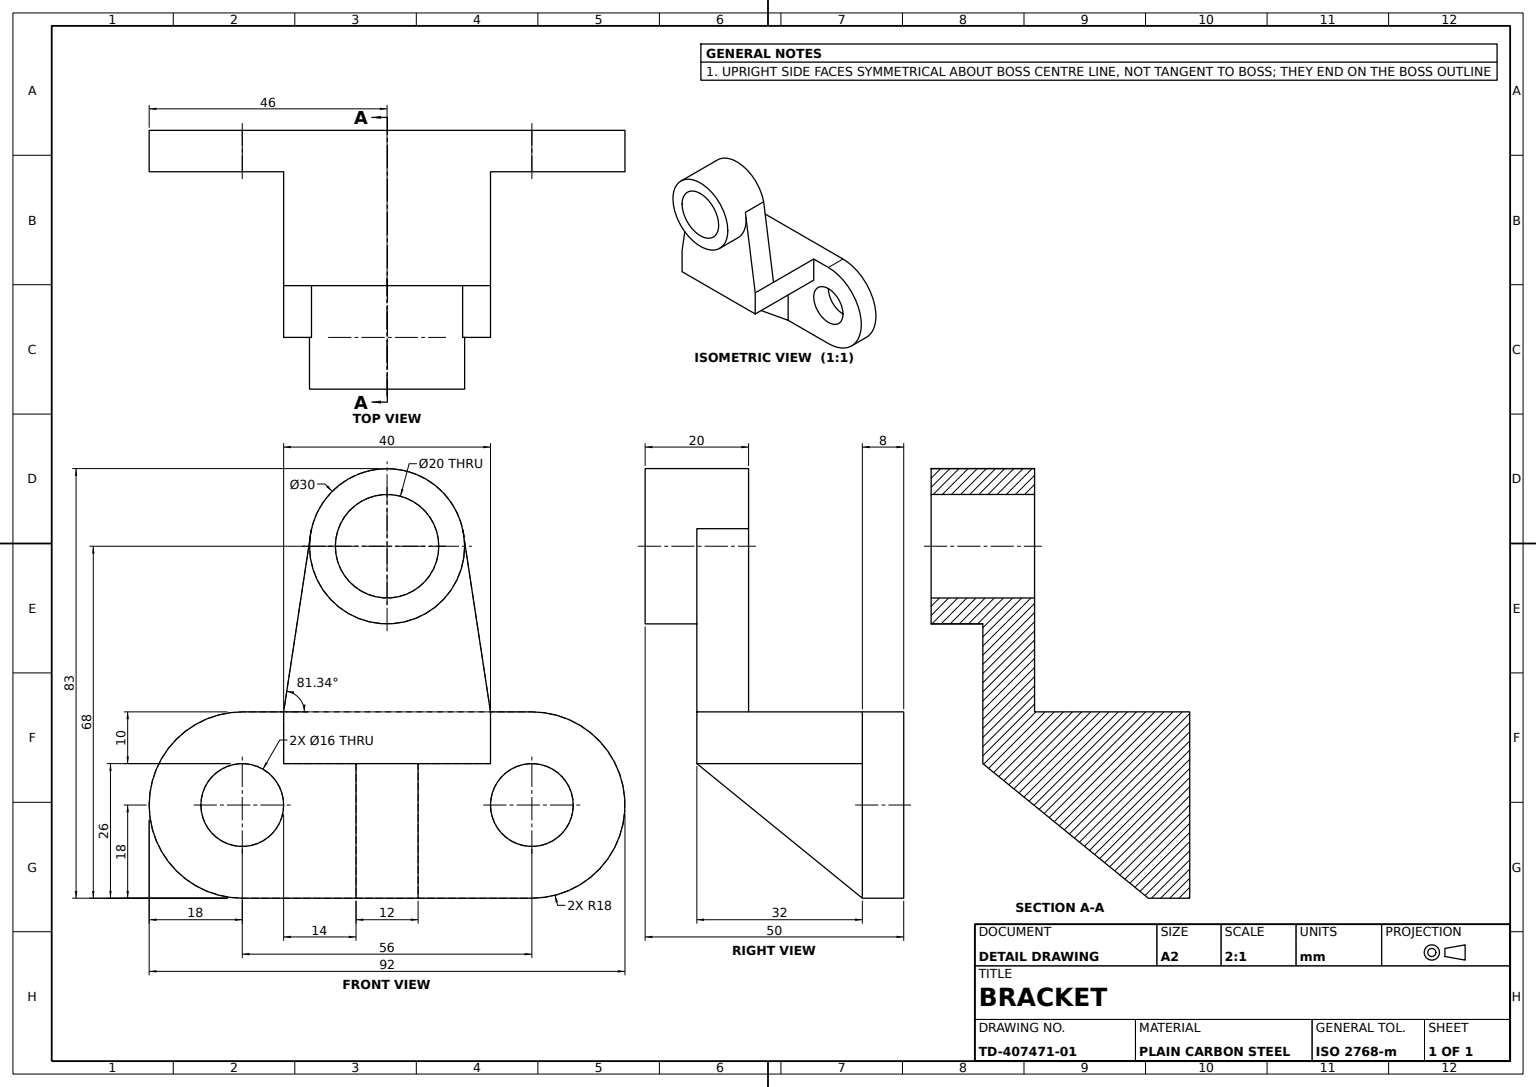
from build123d import *

# Parameters (mm, degrees)
BASE_PLATE_DEPTH       = 8
BASE_HOLE_SKETCH_R     = 8
BASE_HOLE_DEPTH        = 8
UPRIGHT_ARM_DEPTH      = 32
BOSS_MOUNT_DEPTH       = 10
CYLINDER_START         = 10
CYLINDER_BOSS_SKETCH_R = 15
CYLINDER_BOSS_DEPTH    = 10
BOSS_BORE_SKETCH_R     = 10
BOSS_BORE_DEPTH        = 20
GUSSET_DEPTH           = 40
GUSSET_TRIM_1_DEPTH    = 14
GUSSET_TRIM_2_DEPTH    = 14


with BuildPart() as part:
    # Base Plate Sketch → Base Plate (new body)
    with BuildSketch(Plane.XY):
        with BuildLine():
            Line((0, 18), (56, 18))
            ThreePointArc((56, 18), (74, 0), (56, -18))
            Line((56, -18), (0, -18))
            ThreePointArc((0, -18), (-18, 0), (0, 18))
        make_face()
    extrude(amount=BASE_PLATE_DEPTH)

    # Base Hole Sketch → Base Hole (cut)
    with BuildSketch(Plane.XY.offset(8)):
        Circle(BASE_HOLE_SKETCH_R)
        with Locations((56, 0)):
            Circle(BASE_HOLE_SKETCH_R)
    extrude(amount=-BASE_HOLE_DEPTH, mode=Mode.SUBTRACT)

    # Upright Arm Sketch → Upright Arm (add)
    with BuildSketch(Plane.XY.offset(8)):
        Polygon((28, 18), (8, 18), (8, 8), (48, 8), (48, 18), align=None)
    extrude(amount=UPRIGHT_ARM_DEPTH)

    # Boss Mount Sketch → Boss Mount (add)
    with BuildSketch(Plane.XY.offset(40)):
        with BuildLine():
            Line((13.388373349, 53.391219044), (13.041195377, 51.110929457))
            ThreePointArc((13.041195377, 51.110929457), (27.444153502, 35.010302382), (43, 50))
            ThreePointArc((43, 50), (42.989697618, 50.555846498), (42.958804623, 51.110929457))
            Line((42.958804623, 51.110929457), (42.611626651, 53.391219044))
            ThreePointArc((42.611626651, 53.391219044), (28, 65), (13.388373349, 53.391219044))
        make_face()
        with BuildLine():
            Line((13.041195377, 51.110929457), (8, 18))
            Line((8, 18), (48, 18))
            Line((48, 18), (42.958804623, 51.110929457))
            ThreePointArc((42.958804623, 51.110929457), (42.989697618, 50.555846498), (43, 50))
            ThreePointArc((43, 50), (27.444153502, 35.010302382), (13.041195377, 51.110929457))
        make_face()
    extrude(amount=-BOSS_MOUNT_DEPTH)

    # Cylinder Boss Sketch → Cylinder Boss (add)
    with BuildSketch(Plane.XY.offset(40).offset(CYLINDER_START)):
        with Locations((28, 50)):
            Circle(CYLINDER_BOSS_SKETCH_R)
    extrude(amount=-CYLINDER_BOSS_DEPTH)

    # Boss Bore Sketch → Boss Bore (cut)
    with BuildSketch(Plane.XY.offset(50)):
        with Locations((28, 50)):
            Circle(BOSS_BORE_SKETCH_R)
    extrude(amount=-BOSS_BORE_DEPTH, mode=Mode.SUBTRACT)

    # Gusset Sketch → Gusset (add)
    with BuildSketch(Plane(origin=(48, 0, 0), x_dir=(0, 0, -1), z_dir=(1, 0, 0))):
        Polygon((-40, 8), (-8, -18), (-8, 8), align=None)
    extrude(amount=-GUSSET_DEPTH)

    # Gusset Trim 1 Sketch → Gusset Trim 1 (cut)
    with BuildSketch(Plane(origin=(48, 0, 0), x_dir=(0, 0, -1), z_dir=(1, 0, 0))):
        Polygon((-40, 8), (-8, 8), (-8, -18), align=None)
    extrude(amount=-GUSSET_TRIM_1_DEPTH, mode=Mode.SUBTRACT)

    # Gusset Trim 2 Sketch → Gusset Trim 2 (cut)
    with BuildSketch(Plane.ZY.offset(-8)):
        Polygon((40, 8), (8, 8), (8, -18), align=None)
    extrude(amount=-GUSSET_TRIM_2_DEPTH, mode=Mode.SUBTRACT)


solid = part.part
